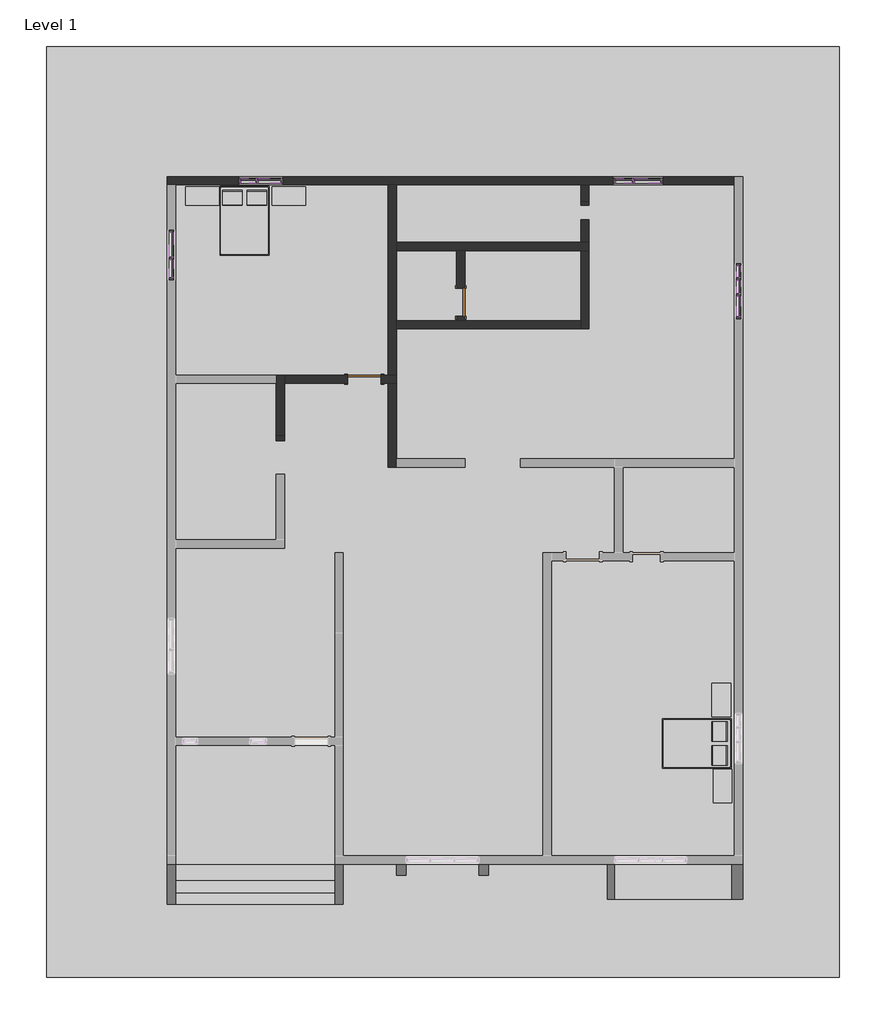
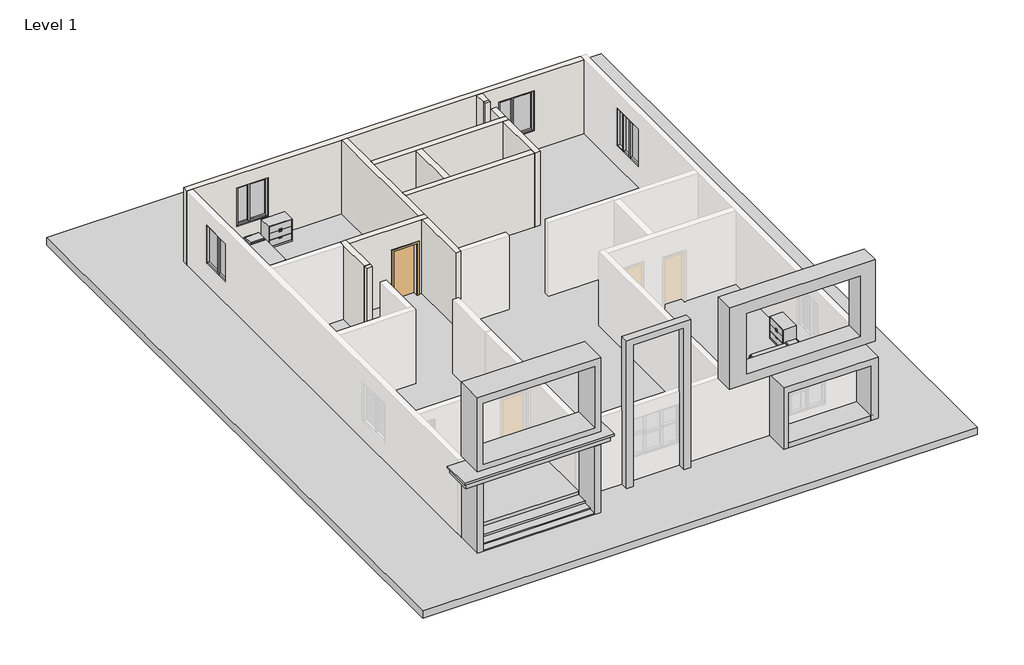
# One storey, part 3 of 3: 31 members, 13 walls, 9 plates, 6 furniture elements, 3 proxies, 2 doors.
"""IFC4 building model written with IfcOpenShell, lengths in millimetres."""

from ifc_helpers import new_model, si_unit, frame, origin, origin_with_axes, place, context, project, spatial, polyline, outline, extrude, faceted_brep, transform, mapped, element, save
from components import generic_models_1_generic_models_1_3e26791c, generic_models_2_generic_models_2_3b55f561, generic_models_3_generic_models_3_0a189295, door_a1484949, door_0ca8825f, furniture_b58f7881, furniture_dccb195e, member_6f432376, member_b9f3750b, member_83c59054, member_02b8d6b6, member_8456be0a, member_cf38170e, member_5535eeb3, member_7007ad49, member_f01f4494, member_224a2a57, member_3f0e0172, member_dc106669, member_0b703233, member_623289aa, member_5f1d7e17, member_11644e99, member_f1c24713, system_panel_glazed_ed2eb233, system_panel_glazed_a8d9a87a, system_panel_glazed_d172bbbe, system_panel_glazed_c29ca9bc, system_panel_glazed_863e5c36, system_panel_glazed_5eb5e9ea, system_panel_glazed_fad1f0ba, system_panel_glazed_bca51d21, system_panel_glazed_cf012afc

model = new_model("IFC4")

# Units and contexts
model_context = context("Model", 3, world=origin())
ifc_project = project(units=[si_unit("LENGTHUNIT", "METRE", prefix="MILLI")], contexts=[model_context])

# Site, building, storey
site = spatial("IfcSite", under=ifc_project)
building = spatial("IfcBuilding", under=site)
storey = spatial("IfcBuildingStorey", under=building, Name="Level 1", Elevation=0.0)

# Proxies
placement = place(None, origin())
generic_models_1_generic_models_1_shape = generic_models_1_generic_models_1_3e26791c(model_context)
element("IfcBuildingElementProxy", 1, Name="Generic Models 1 : Generic Models 1", ObjectType="Generic Models 1 : Generic Models 1", at=placement, inside=storey, context=model_context, shape_type="MappedRepresentation", body=[
    mapped(generic_models_1_generic_models_1_shape, transform((0.0, 0.0, 0.0), x_axis=(1.0, 0.0, 0.0), y_axis=(0.0, 1.0, 0.0), z_axis=(0.0, 0.0, 1.0))),
])
generic_models_2_generic_models_2_shape = generic_models_2_generic_models_2_3b55f561(model_context)
element("IfcBuildingElementProxy", 2, Name="Generic Models 2 : Generic Models 2", ObjectType="Generic Models 2 : Generic Models 2", at=placement, inside=storey, context=model_context, shape_type="MappedRepresentation", body=[
    mapped(generic_models_2_generic_models_2_shape, transform((0.0, 0.0, 0.0), x_axis=(1.0, 0.0, 0.0), y_axis=(0.0, 1.0, 0.0), z_axis=(0.0, 0.0, 1.0))),
])
generic_models_3_generic_models_3_shape = generic_models_3_generic_models_3_0a189295(model_context)
element("IfcBuildingElementProxy", 3, Name="Generic Models 3 : Generic Models 3", ObjectType="Generic Models 3 : Generic Models 3", at=placement, inside=storey, context=model_context, shape_type="MappedRepresentation", body=[
    mapped(generic_models_3_generic_models_3_shape, transform((0.0, 0.0, 0.0), x_axis=(1.0, 0.0, 0.0), y_axis=(0.0, 1.0, 0.0), z_axis=(0.0, 0.0, 1.0))),
])

# Doors
door_shape = door_a1484949(model_context)
element("IfcDoor", 4, ObjectType="Single-Flush : 30\" x 80\"", at=placement, inside=storey, context=model_context, shape_type="MappedRepresentation", body=[
    mapped(door_shape, transform((-11084.7702714, 3728.4616097, 0.0), x_axis=(0.0, -1.0, 0.0), y_axis=(1.0, 0.0, 0.0), z_axis=(0.0, 0.0, 1.0))),
])
door_2_shape = door_0ca8825f(model_context)
element("IfcDoor", 5, ObjectType="Single-Flush : 36\" x 84\"", at=placement, inside=storey, context=model_context, shape_type="MappedRepresentation", body=[
    mapped(door_2_shape, transform((-13713.6702714, 1632.9616097, 0.0), x_axis=(1.0, 0.0, 0.0), y_axis=(0.0, 1.0, 0.0), z_axis=(0.0, 0.0, 1.0))),
])

# Furniture
furniture_shape = furniture_b58f7881(model_context)
element("IfcFurniture", 6, ObjectType="Bed-Box : Double 53\" x 74\"", at=placement, inside=storey, context=model_context, shape_type="MappedRepresentation", body=[
    mapped(furniture_shape, transform((-17316.7227304, 6185.3911179, 0.0), x_axis=(1.0, 0.0, 0.0), y_axis=(0.0, 1.0, 0.0), z_axis=(0.0, 0.0, 1.0))),
])
element("IfcFurniture", 7, ObjectType="Bed-Box : Double 53\" x 74\"", at=placement, inside=storey, context=model_context, shape_type="MappedRepresentation", body=[
    mapped(furniture_shape, transform((-4411.4407632, -7959.2859313, 0.0), x_axis=(0.0, -1.0, 0.0), y_axis=(1.0, 0.0, 0.0), z_axis=(0.0, 0.0, 1.0))),
])
furniture_2_shape = furniture_dccb195e(model_context)
element("IfcFurniture", 8, ObjectType="Cabinet File-Lateral 3 Drawer : 36\" x 20\" x 36\"", at=placement, inside=storey, context=model_context, shape_type="MappedRepresentation", body=[
    mapped(furniture_2_shape, transform((-3038.4518953, -7284.6609042, 0.0), x_axis=(0.0, -1.0, 0.0), y_axis=(1.0, 0.0, 0.0), z_axis=(0.0, 0.0, 1.0))),
])
element("IfcFurniture", 9, ObjectType="Cabinet File-Lateral 3 Drawer : 36\" x 20\" x 36\"", at=placement, inside=storey, context=model_context, shape_type="MappedRepresentation", body=[
    mapped(furniture_2_shape, transform((-3000.3518953, -9634.1609042, 0.0), x_axis=(0.0, -1.0, 0.0), y_axis=(1.0, 0.0, 0.0), z_axis=(0.0, 0.0, 1.0))),
])
element("IfcFurniture", 10, ObjectType="Cabinet File-Lateral 3 Drawer : 36\" x 20\" x 36\"", at=placement, inside=storey, context=model_context, shape_type="MappedRepresentation", body=[
    mapped(furniture_2_shape, transform((-15591.0477575, 7558.3799858, 0.0), x_axis=(1.0, 0.0, 0.0), y_axis=(0.0, 1.0, 0.0), z_axis=(0.0, 0.0, 1.0))),
])
element("IfcFurniture", 11, ObjectType="Cabinet File-Lateral 3 Drawer : 36\" x 20\" x 36\"", at=placement, inside=storey, context=model_context, shape_type="MappedRepresentation", body=[
    mapped(furniture_2_shape, transform((-17953.2477575, 7558.3799858, 0.0), x_axis=(1.0, 0.0, 0.0), y_axis=(0.0, 1.0, 0.0), z_axis=(0.0, 0.0, 1.0))),
])

# Members
member_shape = member_6f432376(model_context)
element("IfcMember", 12, ObjectType="Rectangular Mullion : 2.5\" x 5\" rectangular", at=placement, inside=storey, context=model_context, shape_type="MappedRepresentation", body=[
    mapped(member_shape, transform((-3502.8702714, 3334.7616097, 2404.522235), x_axis=(0.0, 0.0, 1.0), y_axis=(-1.0, 0.0, 0.0), z_axis=(0.0, -1.0, 0.0))),
])
element("IfcMember", 13, ObjectType="Rectangular Mullion : 2.5\" x 5\" rectangular", at=placement, inside=storey, context=model_context, shape_type="MappedRepresentation", body=[
    mapped(member_shape, transform((-3502.8702714, 3899.9116097, 784.7381643), x_axis=(0.0, 0.0, -1.0), y_axis=(-1.0, 0.0, 0.0), z_axis=(0.0, 1.0, 0.0))),
])
member_2_shape = member_b9f3750b(model_context)
element("IfcMember", 14, ObjectType="Rectangular Mullion : 2.5\" x 5\" rectangular", at=placement, inside=storey, context=model_context, shape_type="MappedRepresentation", body=[
    mapped(member_2_shape, transform((-18971.4702714, 4890.5116097, 810.1702203), x_axis=(0.0, 0.0, -1.0), y_axis=(-1.0, 0.0, 0.0), z_axis=(0.0, 1.0, 0.0))),
])
element("IfcMember", 15, ObjectType="Rectangular Mullion : 2.5\" x 5\" rectangular", at=placement, inside=storey, context=model_context, shape_type="MappedRepresentation", body=[
    mapped(member_2_shape, transform((-18971.4702714, 4401.5616097, 2441.6213003), x_axis=(0.0, 0.0, 1.0), y_axis=(-1.0, 0.0, 0.0), z_axis=(0.0, -1.0, 0.0))),
])
member_3_shape = member_83c59054(model_context)
element("IfcMember", 16, ObjectType="Rectangular Mullion : 2.5\" x 5\" rectangular", at=placement, inside=storey, context=model_context, shape_type="MappedRepresentation", body=[
    mapped(member_3_shape, transform((-3502.8702714, 4331.7116097, 784.7381643), x_axis=(0.0, 0.0, -1.0), y_axis=(-1.0, 0.0, 0.0), z_axis=(0.0, 1.0, 0.0))),
])
member_4_shape = member_02b8d6b6(model_context)
element("IfcMember", 17, ObjectType="Rectangular Mullion : 2.5\" x 5\" rectangular", at=placement, inside=storey, context=model_context, shape_type="MappedRepresentation", body=[
    mapped(member_4_shape, transform((-3502.8702714, 4731.7616097, 784.7381643), x_axis=(0.0, 0.0, -1.0), y_axis=(-1.0, 0.0, 0.0), z_axis=(0.0, 1.0, 0.0))),
])
member_5_shape = member_8456be0a(model_context)
element("IfcMember", 18, ObjectType="Rectangular Mullion : 2.5\" x 5\" rectangular", at=placement, inside=storey, context=model_context, shape_type="MappedRepresentation", body=[
    mapped(member_5_shape, transform((-3502.8702714, 3931.6616097, 784.7381643), x_axis=(0.0, -1.0, 0.0), y_axis=(-1.0, 0.0, 0.0), z_axis=(0.0, 0.0, -1.0))),
])
element("IfcMember", 19, ObjectType="Rectangular Mullion : 2.5\" x 5\" rectangular", at=placement, inside=storey, context=model_context, shape_type="MappedRepresentation", body=[
    mapped(member_5_shape, transform((-3502.8702714, 4363.4616097, 784.7381643), x_axis=(0.0, -1.0, 0.0), y_axis=(-1.0, 0.0, 0.0), z_axis=(0.0, 0.0, -1.0))),
])
element("IfcMember", 20, ObjectType="Rectangular Mullion : 2.5\" x 5\" rectangular", at=placement, inside=storey, context=model_context, shape_type="MappedRepresentation", body=[
    mapped(member_4_shape, transform((-3502.8702714, 4395.2116097, 2404.522235), x_axis=(0.0, 0.0, 1.0), y_axis=(-1.0, 0.0, 0.0), z_axis=(0.0, -1.0, 0.0))),
])
element("IfcMember", 21, ObjectType="Rectangular Mullion : 2.5\" x 5\" rectangular", at=placement, inside=storey, context=model_context, shape_type="MappedRepresentation", body=[
    mapped(member_3_shape, transform((-3502.8702714, 3963.4116097, 2404.522235), x_axis=(0.0, 0.0, 1.0), y_axis=(-1.0, 0.0, 0.0), z_axis=(0.0, -1.0, 0.0))),
])
member_6_shape = member_cf38170e(model_context)
element("IfcMember", 22, ObjectType="Rectangular Mullion : 2.5\" x 5\" rectangular", at=placement, inside=storey, context=model_context, shape_type="MappedRepresentation", body=[
    mapped(member_6_shape, transform((-3502.8702714, 4795.2616097, 2404.522235), x_axis=(0.0, 1.0, 0.0), y_axis=(-1.0, 0.0, 0.0), z_axis=(0.0, 0.0, 1.0))),
])
element("IfcMember", 23, ObjectType="Rectangular Mullion : 2.5\" x 5\" rectangular", at=placement, inside=storey, context=model_context, shape_type="MappedRepresentation", body=[
    mapped(member_6_shape, transform((-3502.8702714, 3271.2616097, 784.7381643), x_axis=(0.0, -1.0, 0.0), y_axis=(-1.0, 0.0, 0.0), z_axis=(0.0, 0.0, -1.0))),
])
member_7_shape = member_5535eeb3(model_context)
element("IfcMember", 24, ObjectType="Rectangular Mullion : 2.5\" x 5\" rectangular", at=placement, inside=storey, context=model_context, shape_type="MappedRepresentation", body=[
    mapped(member_7_shape, transform((-6404.8202714, 7043.1616097, 2451.8488146), x_axis=(0.0, 0.0, 1.0), y_axis=(0.0, -1.0, 0.0), z_axis=(1.0, 0.0, 0.0))),
])
member_8_shape = member_7007ad49(model_context)
element("IfcMember", 25, ObjectType="Rectangular Mullion : 2.5\" x 5\" rectangular", at=placement, inside=storey, context=model_context, shape_type="MappedRepresentation", body=[
    mapped(member_8_shape, transform((-5623.7702714, 7043.1616097, 2451.8488146), x_axis=(0.0, 0.0, 1.0), y_axis=(0.0, -1.0, 0.0), z_axis=(1.0, 0.0, 0.0))),
])
member_9_shape = member_f01f4494(model_context)
element("IfcMember", 26, ObjectType="Rectangular Mullion : 2.5\" x 5\" rectangular", at=placement, inside=storey, context=model_context, shape_type="MappedRepresentation", body=[
    mapped(member_9_shape, transform((-6373.0702714, 7043.1616097, 795.4375908), x_axis=(1.0, 0.0, 0.0), y_axis=(0.0, -1.0, 0.0), z_axis=(0.0, 0.0, -1.0))),
])
element("IfcMember", 27, ObjectType="Rectangular Mullion : 2.5\" x 5\" rectangular", at=placement, inside=storey, context=model_context, shape_type="MappedRepresentation", body=[
    mapped(member_8_shape, transform((-6341.3202714, 7043.1616097, 795.4375908), x_axis=(0.0, 0.0, -1.0), y_axis=(0.0, -1.0, 0.0), z_axis=(-1.0, 0.0, 0.0))),
])
element("IfcMember", 28, ObjectType="Rectangular Mullion : 2.5\" x 5\" rectangular", at=placement, inside=storey, context=model_context, shape_type="MappedRepresentation", body=[
    mapped(member_7_shape, transform((-6868.3702714, 7043.1616097, 795.4375908), x_axis=(0.0, 0.0, -1.0), y_axis=(0.0, -1.0, 0.0), z_axis=(-1.0, 0.0, 0.0))),
])
member_10_shape = member_224a2a57(model_context)
element("IfcMember", 29, ObjectType="Rectangular Mullion : 2.5\" x 5\" rectangular", at=placement, inside=storey, context=model_context, shape_type="MappedRepresentation", body=[
    mapped(member_10_shape, transform((-6931.8702714, 7043.1616097, 2451.8488146), x_axis=(-1.0, 0.0, 0.0), y_axis=(0.0, -1.0, 0.0), z_axis=(0.0, 0.0, 1.0))),
])
element("IfcMember", 30, ObjectType="Rectangular Mullion : 2.5\" x 5\" rectangular", at=placement, inside=storey, context=model_context, shape_type="MappedRepresentation", body=[
    mapped(member_10_shape, transform((-5560.2702714, 7043.1616097, 795.4375908), x_axis=(1.0, 0.0, 0.0), y_axis=(0.0, -1.0, 0.0), z_axis=(0.0, 0.0, -1.0))),
])
member_11_shape = member_3f0e0172(model_context)
element("IfcMember", 31, ObjectType="Rectangular Mullion : 2.5\" x 5\" rectangular", at=placement, inside=storey, context=model_context, shape_type="MappedRepresentation", body=[
    mapped(member_11_shape, transform((-16602.9202714, 7043.1616097, 907.4058093), x_axis=(0.0, 0.0, -1.0), y_axis=(0.0, -1.0, 0.0), z_axis=(-1.0, 0.0, 0.0))),
])
member_12_shape = member_dc106669(model_context)
element("IfcMember", 32, ObjectType="Rectangular Mullion : 2.5\" x 5\" rectangular", at=placement, inside=storey, context=model_context, shape_type="MappedRepresentation", body=[
    mapped(member_12_shape, transform((-17079.1702714, 7043.1616097, 907.4058093), x_axis=(0.0, 0.0, -1.0), y_axis=(0.0, -1.0, 0.0), z_axis=(-1.0, 0.0, 0.0))),
])
member_13_shape = member_0b703233(model_context)
element("IfcMember", 33, ObjectType="Rectangular Mullion : 2.5\" x 5\" rectangular", at=placement, inside=storey, context=model_context, shape_type="MappedRepresentation", body=[
    mapped(member_13_shape, transform((-16634.6702714, 7043.1616097, 907.4058093), x_axis=(1.0, 0.0, 0.0), y_axis=(0.0, -1.0, 0.0), z_axis=(0.0, 0.0, -1.0))),
])
element("IfcMember", 34, ObjectType="Rectangular Mullion : 2.5\" x 5\" rectangular", at=placement, inside=storey, context=model_context, shape_type="MappedRepresentation", body=[
    mapped(member_12_shape, transform((-16666.4202714, 7043.1616097, 2493.6914356), x_axis=(0.0, 0.0, 1.0), y_axis=(0.0, -1.0, 0.0), z_axis=(1.0, 0.0, 0.0))),
])
element("IfcMember", 35, ObjectType="Rectangular Mullion : 2.5\" x 5\" rectangular", at=placement, inside=storey, context=model_context, shape_type="MappedRepresentation", body=[
    mapped(member_11_shape, transform((-15986.9702714, 7043.1616097, 2493.6914356), x_axis=(0.0, 0.0, 1.0), y_axis=(0.0, -1.0, 0.0), z_axis=(1.0, 0.0, 0.0))),
])
member_14_shape = member_623289aa(model_context)
element("IfcMember", 36, ObjectType="Rectangular Mullion : 2.5\" x 5\" rectangular", at=placement, inside=storey, context=model_context, shape_type="MappedRepresentation", body=[
    mapped(member_14_shape, transform((-17142.6702714, 7043.1616097, 2493.6914356), x_axis=(-1.0, 0.0, 0.0), y_axis=(0.0, -1.0, 0.0), z_axis=(0.0, 0.0, 1.0))),
])
element("IfcMember", 37, ObjectType="Rectangular Mullion : 2.5\" x 5\" rectangular", at=placement, inside=storey, context=model_context, shape_type="MappedRepresentation", body=[
    mapped(member_14_shape, transform((-15923.4702714, 7043.1616097, 907.4058093), x_axis=(1.0, 0.0, 0.0), y_axis=(0.0, -1.0, 0.0), z_axis=(0.0, 0.0, -1.0))),
])
member_15_shape = member_5f1d7e17(model_context)
element("IfcMember", 38, ObjectType="Rectangular Mullion : 2.5\" x 5\" rectangular", at=placement, inside=storey, context=model_context, shape_type="MappedRepresentation", body=[
    mapped(member_15_shape, transform((-18971.4702714, 4954.0116097, 2441.6213003), x_axis=(0.0, 0.0, 1.0), y_axis=(-1.0, 0.0, 0.0), z_axis=(0.0, -1.0, 0.0))),
])
member_16_shape = member_11644e99(model_context)
element("IfcMember", 39, ObjectType="Rectangular Mullion : 2.5\" x 5\" rectangular", at=placement, inside=storey, context=model_context, shape_type="MappedRepresentation", body=[
    mapped(member_16_shape, transform((-18971.4702714, 4922.2616097, 810.1702203), x_axis=(0.0, -1.0, 0.0), y_axis=(-1.0, 0.0, 0.0), z_axis=(0.0, 0.0, -1.0))),
])
element("IfcMember", 40, ObjectType="Rectangular Mullion : 2.5\" x 5\" rectangular", at=placement, inside=storey, context=model_context, shape_type="MappedRepresentation", body=[
    mapped(member_15_shape, transform((-18971.4702714, 5646.1616097, 810.1702203), x_axis=(0.0, 0.0, -1.0), y_axis=(-1.0, 0.0, 0.0), z_axis=(0.0, 1.0, 0.0))),
])
member_17_shape = member_f1c24713(model_context)
element("IfcMember", 41, ObjectType="Rectangular Mullion : 2.5\" x 5\" rectangular", at=placement, inside=storey, context=model_context, shape_type="MappedRepresentation", body=[
    mapped(member_17_shape, transform((-18971.4702714, 4338.0616097, 810.1702203), x_axis=(0.0, -1.0, 0.0), y_axis=(-1.0, 0.0, 0.0), z_axis=(0.0, 0.0, -1.0))),
])
element("IfcMember", 42, ObjectType="Rectangular Mullion : 2.5\" x 5\" rectangular", at=placement, inside=storey, context=model_context, shape_type="MappedRepresentation", body=[
    mapped(member_17_shape, transform((-18971.4702714, 5709.6616097, 2441.6213003), x_axis=(0.0, 1.0, 0.0), y_axis=(-1.0, 0.0, 0.0), z_axis=(0.0, 0.0, 1.0))),
])

# Plates
system_panel_glazed_shape = system_panel_glazed_ed2eb233(model_context)
element("IfcPlate", 43, ObjectType="System Panel : Glazed", at=placement, inside=storey, context=model_context, shape_type="MappedRepresentation", body=[
    mapped(system_panel_glazed_shape, transform((-3502.8702714, 4563.4866097, 848.2381643), x_axis=(0.0, -1.0, 0.0), y_axis=(1.0, 0.0, 0.0), z_axis=(0.0, 0.0, 1.0))),
])
system_panel_glazed_2_shape = system_panel_glazed_a8d9a87a(model_context)
element("IfcPlate", 44, ObjectType="System Panel : Glazed", at=placement, inside=storey, context=model_context, shape_type="MappedRepresentation", body=[
    mapped(system_panel_glazed_2_shape, transform((-3502.8702714, 3617.3366097, 848.2381643), x_axis=(0.0, -1.0, 0.0), y_axis=(1.0, 0.0, 0.0), z_axis=(0.0, 0.0, 1.0))),
])
system_panel_glazed_3_shape = system_panel_glazed_d172bbbe(model_context)
element("IfcPlate", 45, ObjectType="System Panel : Glazed", at=placement, inside=storey, context=model_context, shape_type="MappedRepresentation", body=[
    mapped(system_panel_glazed_3_shape, transform((-3502.8702714, 4147.5616097, 848.2381643), x_axis=(0.0, -1.0, 0.0), y_axis=(1.0, 0.0, 0.0), z_axis=(0.0, 0.0, 1.0))),
])
system_panel_glazed_4_shape = system_panel_glazed_c29ca9bc(model_context)
element("IfcPlate", 46, ObjectType="System Panel : Glazed", at=placement, inside=storey, context=model_context, shape_type="MappedRepresentation", body=[
    mapped(system_panel_glazed_4_shape, transform((-6636.5952714, 7043.1616097, 858.9375908), x_axis=(1.0, 0.0, 0.0), y_axis=(0.0, 1.0, 0.0), z_axis=(0.0, 0.0, 1.0))),
])
system_panel_glazed_5_shape = system_panel_glazed_863e5c36(model_context)
element("IfcPlate", 47, ObjectType="System Panel : Glazed", at=placement, inside=storey, context=model_context, shape_type="MappedRepresentation", body=[
    mapped(system_panel_glazed_5_shape, transform((-5982.5452714, 7043.1616097, 858.9375908), x_axis=(1.0, 0.0, 0.0), y_axis=(0.0, 1.0, 0.0), z_axis=(0.0, 0.0, 1.0))),
])
system_panel_glazed_6_shape = system_panel_glazed_5eb5e9ea(model_context)
element("IfcPlate", 48, ObjectType="System Panel : Glazed", at=placement, inside=storey, context=model_context, shape_type="MappedRepresentation", body=[
    mapped(system_panel_glazed_6_shape, transform((-16872.7952714, 7043.1616097, 970.9058093), x_axis=(1.0, 0.0, 0.0), y_axis=(0.0, 1.0, 0.0), z_axis=(0.0, 0.0, 1.0))),
])
system_panel_glazed_7_shape = system_panel_glazed_fad1f0ba(model_context)
element("IfcPlate", 49, ObjectType="System Panel : Glazed", at=placement, inside=storey, context=model_context, shape_type="MappedRepresentation", body=[
    mapped(system_panel_glazed_7_shape, transform((-16294.9452714, 7043.1616097, 970.9058093), x_axis=(1.0, 0.0, 0.0), y_axis=(0.0, 1.0, 0.0), z_axis=(0.0, 0.0, 1.0))),
])
system_panel_glazed_8_shape = system_panel_glazed_bca51d21(model_context)
element("IfcPlate", 50, ObjectType="System Panel : Glazed", at=placement, inside=storey, context=model_context, shape_type="MappedRepresentation", body=[
    mapped(system_panel_glazed_8_shape, transform((-18971.4702714, 5300.0866097, 873.6702203), x_axis=(0.0, -1.0, 0.0), y_axis=(1.0, 0.0, 0.0), z_axis=(0.0, 0.0, 1.0))),
])
system_panel_glazed_9_shape = system_panel_glazed_cf012afc(model_context)
element("IfcPlate", 51, ObjectType="System Panel : Glazed", at=placement, inside=storey, context=model_context, shape_type="MappedRepresentation", body=[
    mapped(system_panel_glazed_9_shape, transform((-18971.4702714, 4646.0366097, 873.6702203), x_axis=(0.0, -1.0, 0.0), y_axis=(1.0, 0.0, 0.0), z_axis=(0.0, 0.0, 1.0))),
])

# Walls
element("IfcWall", 52, ObjectType="9\"", at=placement, inside=storey, context=model_context, shape_type="Brep", body=[
    faceted_brep([(-3617.1702714, 7157.4616097, 0.0), (-19085.7702714, 7157.4616097, 0.0), (-19085.7702714, 7157.4616097, 3048.0), (-3617.1702714, 7157.4616097, 3048.0), (-6931.8702714, 7157.4616097, 2451.8488146), (-6931.8702714, 7157.4616097, 795.4375908), (-5560.2702714, 7157.4616097, 795.4375908), (-5560.2702714, 7157.4616097, 2451.8488146), (-17142.6702714, 7157.4616097, 2493.6914356), (-17142.6702714, 7157.4616097, 907.4058093), (-15923.4702714, 7157.4616097, 907.4058093), (-15923.4702714, 7157.4616097, 2493.6914356), (-19085.7702714, 6928.8616097, 0.0), (-18857.1702714, 6928.8616097, 0.0), (-13065.9702714, 6928.8616097, 0.0), (-12837.3702714, 6928.8616097, 0.0), (-7808.1702714, 6928.8616097, 0.0), (-7579.5702714, 6928.8616097, 0.0), (-3617.1702714, 6928.8616097, 0.0), (-3617.1702714, 6928.8616097, 3048.0), (-7579.5702714, 6928.8616097, 3048.0), (-7808.1702714, 6928.8616097, 3048.0), (-12837.3702714, 6928.8616097, 3048.0), (-13065.9702714, 6928.8616097, 3048.0), (-18857.1702714, 6928.8616097, 3048.0), (-19085.7702714, 6928.8616097, 3048.0), (-6931.8702714, 6928.8616097, 795.4375908), (-6931.8702714, 6928.8616097, 2451.8488146), (-5560.2702714, 6928.8616097, 2451.8488146), (-5560.2702714, 6928.8616097, 795.4375908), (-17142.6702714, 6928.8616097, 907.4058093), (-17142.6702714, 6928.8616097, 2493.6914356), (-15923.4702714, 6928.8616097, 2493.6914356), (-15923.4702714, 6928.8616097, 907.4058093)], [[[0, 1, 2, 3], [4, 5, 6, 7], [8, 9, 10, 11]], [[12, 13, 14, 15, 16, 17, 18, 19, 20, 21, 22, 23, 24, 25], [26, 27, 28, 29], [30, 31, 32, 33]], [[1, 0, 18, 17, 16, 15, 14, 13, 12]], [[3, 2, 25, 24, 23, 22, 21, 20, 19]], [[0, 3, 19, 18]], [[2, 1, 12, 25]], [[4, 27, 26, 5]], [[27, 4, 7, 28]], [[28, 7, 6, 29]], [[5, 26, 29, 6]], [[30, 9, 8, 31]], [[31, 8, 11, 32]], [[32, 11, 10, 33]], [[9, 30, 33, 10]]]),
])
element("IfcWall", 53, ObjectType="9\"", at=placement, inside=storey, context=model_context, shape_type="Brep", body=[
    faceted_brep([(-13256.4702714, 1518.6616097, 2133.6), (-13256.4702714, 1518.6616097, 0.0), (-13065.9702714, 1518.6616097, 0.0), (-12837.3702714, 1518.6616097, 0.0), (-12837.3702714, 1518.6616097, 3048.0), (-13065.9702714, 1518.6616097, 3048.0), (-15885.3702714, 1518.6616097, 3048.0), (-15885.3702714, 1518.6616097, 0.0), (-14170.8702714, 1518.6616097, 0.0), (-14170.8702714, 1518.6616097, 2133.6), (-12837.3702714, 1747.2616097, 0.0), (-13065.9702714, 1747.2616097, 0.0), (-13256.4702714, 1747.2616097, 0.0), (-13256.4702714, 1747.2616097, 2133.6), (-14170.8702714, 1747.2616097, 2133.6), (-14170.8702714, 1747.2616097, 0.0), (-15885.3702714, 1747.2616097, 0.0), (-15885.3702714, 1747.2616097, 3048.0), (-13065.9702714, 1747.2616097, 3048.0), (-12837.3702714, 1747.2616097, 3048.0)], [[[0, 1, 2, 3, 4, 5, 6, 7, 8, 9]], [[10, 11, 12, 13, 14, 15, 16, 17, 18, 19]], [[8, 7, 16, 15]], [[3, 2, 1, 12, 11, 10]], [[6, 5, 4, 19, 18, 17]], [[7, 6, 17, 16]], [[4, 3, 10, 19]], [[13, 12, 1, 0]], [[14, 13, 0, 9]], [[15, 14, 9, 8]]]),
])
element("IfcWall", 54, ObjectType="9\"", at=placement, inside=storey, context=model_context, shape_type="Brep", body=[
    faceted_brep([(-12837.3702714, 1747.2616097, 0.0), (-12837.3702714, 3004.5616097, 0.0), (-12837.3702714, 3233.1616097, 0.0), (-12837.3702714, 5138.1616097, 0.0), (-12837.3702714, 5366.7616097, 0.0), (-12837.3702714, 6928.8616097, 0.0), (-12837.3702714, 6928.8616097, 3048.0), (-12837.3702714, 5366.7616097, 3048.0), (-12837.3702714, 5138.1616097, 3048.0), (-12837.3702714, 3233.1616097, 3048.0), (-12837.3702714, 3004.5616097, 3048.0), (-12837.3702714, 1747.2616097, 3048.0), (-13065.9702714, 1747.2616097, 0.0), (-13065.9702714, 1747.2616097, 3048.0), (-13065.9702714, 6928.8616097, 3048.0), (-13065.9702714, 6928.8616097, 0.0)], [[[0, 1, 2, 3, 4, 5, 6, 7, 8, 9, 10, 11]], [[12, 13, 14, 15]], [[5, 4, 3, 2, 1, 0, 12, 15]], [[11, 10, 9, 8, 7, 6, 14, 13]], [[0, 11, 13, 12]], [[6, 5, 15, 14]]]),
])
element("IfcWall", 55, ObjectType="9\"", at=placement, inside=storey, context=model_context, shape_type="Brep", body=[
    faceted_brep([(-12837.3702714, 5138.1616097, 0.0), (-11199.0702714, 5138.1616097, 0.0), (-10970.4702714, 5138.1616097, 0.0), (-7808.1702714, 5138.1616097, 0.0), (-7579.5702714, 5138.1616097, 0.0), (-7579.5702714, 5138.1616097, 3048.0), (-7808.1702714, 5138.1616097, 3048.0), (-10970.4702714, 5138.1616097, 3048.0), (-11199.0702714, 5138.1616097, 3048.0), (-12837.3702714, 5138.1616097, 3048.0), (-12837.3702714, 5366.7616097, 0.0), (-12837.3702714, 5366.7616097, 3048.0), (-7808.1702714, 5366.7616097, 3048.0), (-7579.5702714, 5366.7616097, 3048.0), (-7579.5702714, 5366.7616097, 0.0), (-7808.1702714, 5366.7616097, 0.0)], [[[0, 1, 2, 3, 4, 5, 6, 7, 8, 9]], [[10, 11, 12, 13, 14, 15]], [[4, 3, 2, 1, 0, 10, 15, 14]], [[9, 8, 7, 6, 5, 13, 12, 11]], [[0, 9, 11, 10]], [[5, 4, 14, 13]]]),
])
element("IfcWall", 56, ObjectType="9\"", at=placement, inside=storey, context=model_context, shape_type="SweptSolid", body=[
    extrude(outline(polyline([(-7579.5702714, 5976.3616097), (-7579.5702714, 5366.7616097), (-7808.1702714, 5366.7616097), (-7808.1702714, 5976.3616097), (-7579.5702714, 5976.3616097)])), origin_with_axes(), (0.0, 0.0, 1.0), 3048.0),
])
element("IfcWall", 57, ObjectType="9\"", at=placement, inside=storey, context=model_context, shape_type="Brep", body=[
    faceted_brep([(-13065.9702714, 1518.6616097, 0.0), (-13065.9702714, -767.3383903, 0.0), (-13065.9702714, -767.3383903, 3048.0), (-13065.9702714, 1518.6616097, 3048.0), (-12837.3702714, 1518.6616097, 0.0), (-12837.3702714, 1518.6616097, 3048.0), (-12837.3702714, -538.7383903, 3048.0), (-12837.3702714, -767.3383903, 3048.0), (-12837.3702714, -767.3383903, 0.0), (-12837.3702714, -538.7383903, 0.0)], [[[0, 1, 2, 3]], [[4, 5, 6, 7, 8, 9]], [[1, 0, 4, 9, 8]], [[3, 2, 7, 6, 5]], [[0, 3, 5, 4]], [[2, 1, 8, 7]]]),
])
element("IfcWall", 58, ObjectType="9\"", at=placement, inside=storey, context=model_context, shape_type="Brep", body=[
    faceted_brep([(-7808.1702714, 5138.1616097, 0.0), (-7808.1702714, 3233.1616097, 0.0), (-7808.1702714, 3004.5616097, 0.0), (-7808.1702714, 3004.5616097, 3048.0), (-7808.1702714, 3233.1616097, 3048.0), (-7808.1702714, 5138.1616097, 3048.0), (-7579.5702714, 5138.1616097, 0.0), (-7579.5702714, 5138.1616097, 3048.0), (-7579.5702714, 3004.5616097, 3048.0), (-7579.5702714, 3004.5616097, 0.0)], [[[0, 1, 2, 3, 4, 5]], [[6, 7, 8, 9]], [[2, 1, 0, 6, 9]], [[5, 4, 3, 8, 7]], [[0, 5, 7, 6]], [[3, 2, 9, 8]]]),
])
element("IfcWall", 59, ObjectType="9\"", at=placement, inside=storey, context=model_context, shape_type="Brep", body=[
    faceted_brep([(-7808.1702714, 3233.1616097, 0.0), (-10970.4702714, 3233.1616097, 0.0), (-11199.0702714, 3233.1616097, 0.0), (-12837.3702714, 3233.1616097, 0.0), (-12837.3702714, 3233.1616097, 3048.0), (-11199.0702714, 3233.1616097, 3048.0), (-10970.4702714, 3233.1616097, 3048.0), (-7808.1702714, 3233.1616097, 3048.0), (-7808.1702714, 3004.5616097, 0.0), (-7808.1702714, 3004.5616097, 3048.0), (-12837.3702714, 3004.5616097, 3048.0), (-12837.3702714, 3004.5616097, 0.0)], [[[0, 1, 2, 3, 4, 5, 6, 7]], [[8, 9, 10, 11]], [[3, 2, 1, 0, 8, 11]], [[7, 6, 5, 4, 10, 9]], [[0, 7, 9, 8]], [[4, 3, 11, 10]]]),
])
element("IfcWall", 60, ObjectType="9\"", at=placement, inside=storey, context=model_context, shape_type="SweptSolid", body=[
    extrude(outline(polyline([(3347.4616097, 2032.0), (3347.4616097, 0.0), (3233.1616097, 0.0), (3233.1616097, 3048.0), (5138.1616097, 3048.0), (5138.1616097, 0.0), (4109.4616097, 0.0), (4109.4616097, 2032.0), (3347.4616097, 2032.0)])), frame((-11199.0702714, 0.0, 0.0), z_axis=(1.0, 0.0, 0.0), x_axis=(0.0, 1.0, 0.0)), (0.0, 0.0, 1.0), 228.6),
])
element("IfcWall", 61, ObjectType="9\"", at=placement, inside=storey, context=model_context, shape_type="Brep", body=[
    faceted_brep([(-15885.3702714, 108.9616097, 0.0), (-15885.3702714, 1518.6616097, 0.0), (-15885.3702714, 1747.2616097, 0.0), (-15885.3702714, 1747.2616097, 3048.0), (-15885.3702714, 1518.6616097, 3048.0), (-15885.3702714, 108.9616097, 3048.0), (-16113.9702714, 108.9616097, 0.0), (-16113.9702714, 108.9616097, 3048.0), (-16113.9702714, 1518.6616097, 3048.0), (-16113.9702714, 1747.2616097, 3048.0), (-16113.9702714, 1747.2616097, 0.0), (-16113.9702714, 1518.6616097, 0.0)], [[[0, 1, 2, 3, 4, 5]], [[6, 7, 8, 9, 10, 11]], [[2, 1, 0, 6, 11, 10]], [[5, 4, 3, 9, 8, 7]], [[0, 5, 7, 6]], [[3, 2, 10, 9]]]),
])
element("IfcWall", 62, ObjectType="9\"", at=placement, inside=storey, context=model_context, shape_type="SweptSolid", body=[
    extrude(outline(polyline([(-15885.3702714, 108.9616097), (-15885.3702714, -43.4383903), (-16113.9702714, -43.4383903), (-16113.9702714, 108.9616097), (-15885.3702714, 108.9616097)])), origin_with_axes(), (0.0, 0.0, 1.0), 3048.0),
])
element("IfcWall", 63, ObjectType="9\"", at=placement, inside=storey, context=model_context, shape_type="SweptSolid", body=[
    extrude(outline(polyline([(-7579.5702714, 6928.8616097), (-7579.5702714, 6484.3616097), (-7808.1702714, 6484.3616097), (-7808.1702714, 6928.8616097), (-7579.5702714, 6928.8616097)])), origin_with_axes(), (0.0, 0.0, 1.0), 3048.0),
])
element("IfcWall", 64, ObjectType="9\"", at=placement, inside=storey, context=model_context, shape_type="SweptSolid", body=[
    extrude(outline(polyline([(-7579.5702714, 6484.3616097), (-7579.5702714, 6382.7616097), (-7808.1702714, 6382.7616097), (-7808.1702714, 6484.3616097), (-7579.5702714, 6484.3616097)])), origin_with_axes(), (0.0, 0.0, 1.0), 3048.0),
])

save(model, "model.ifc")

# Revit data of these elements
# Type "Single-Flush : 30\" x 80\""
#   Type Mark = "5"
#   Construction Type Id = "MDOOR"
#   Assembly Code = "C1020"
#   Analytic Construction = "Metal"
#   Thickness = 0' - 2"
#   Heat Transfer Coefficient (U) = 0.651978 BTU/(h·ft²·°F)
#   Height = 6' - 8"
#   Trim Projection Ext = 0' - 1"
#   Trim Projection Int = 0' - 1"
#   Trim Width = 0' - 3"
#   Width = 2' - 6"
#   Define Thermal Properties by = 1
#   Define Thermal Properties by = 1
#   Door Material = Door - Panel
#   Frame Material = Door - Frame
#   Visual Light Transmittance = 0
#   Solar Heat Gain Coefficient = 0
#   Function = (empty or 0)
#   Wall Closure = (empty or 0)
# Type "Single-Flush : 36\" x 84\""
#   Type Mark = "1"
#   Construction Type Id = "MDOOR"
#   Assembly Code = "C1020"
#   Analytic Construction = "Metal"
#   Thickness = 0' - 2"
#   Heat Transfer Coefficient (U) = 0.651978 BTU/(h·ft²·°F)
#   Height = 7' - 0"
#   Trim Projection Ext = 0' - 1"
#   Trim Projection Int = 0' - 1"
#   Trim Width = 0' - 3"
#   Width = 3' - 0"
#   Define Thermal Properties by = 1
#   Define Thermal Properties by = 1
#   Door Material = Door - Panel
#   Frame Material = Door - Frame
#   Visual Light Transmittance = 0
#   Solar Heat Gain Coefficient = 0
#   Function = (empty or 0)
#   Wall Closure = (empty or 0)
# Type "Bed-Box : Double 53\" x 74\""
#   Assembly Code = "E2020200"
#   Length = 6' - 2"
#   Width = 4' - 5"
#   Frame Material = Birch
#   Mattress Material = Linen, White
#   Default Elevation = 0
# Type "Cabinet File-Lateral 3 Drawer : 36\" x 20\" x 36\""
#   Assembly Code = "E2020200"
#   Depth = 1' - 8"
#   Height = 3' - 0"
#   Width = 3' - 0"
#   Material = Metal - Steel
#   Default Elevation = 0
# Type "Rectangular Mullion : 2.5\" x 5\" rectangular"
#   built-in parameter 1007304 = 0.416667 (stored number, unit not read)
#   built-in parameter 1007301 = 0.104167 (stored number, unit not read)
#   built-in parameter 1007300 = 0.104167 (stored number, unit not read)
# Type "System Panel : Glazed"
#   Construction Type Id = "GSP4R"
#   Analytic Construction = "1/8 in Pilkington single glazing"
#   Visual Light Transmittance = 0.9
#   Solar Heat Gain Coefficient = 0.86
#   Heat Transfer Coefficient (U) = 1.18115 BTU/(h·ft²·°F)
#   Define Thermal Properties by = 1
# Type "9\""
#   Assembly Code = "B2010"
#   Layers, outside or top first: 0' - 9" no material (function 1)
# Element 1 (IfcBuildingElementProxy, "Generic Models 1 : Generic Models 1")
#   Phase Created = New Construction
# Element 2 (IfcBuildingElementProxy, "Generic Models 2 : Generic Models 2")
#   Phase Created = New Construction
# Element 3 (IfcBuildingElementProxy, "Generic Models 3 : Generic Models 3")
#   Phase Created = New Construction
# Element 4 (IfcDoor, "Single-Flush : 30\" x 80\"")
#   Phase Created = New Construction
#   Materials on its faces: "Door - Frame", "Door - Panel"
# Element 5 (IfcDoor, "Single-Flush : 36\" x 84\"")
#   Phase Created = New Construction
#   Materials on its faces: "Door - Frame", "Door - Panel"
# Elements 6, 7 (IfcFurniture, "Bed-Box : Double 53\" x 74\"")
#   Phase Created = New Construction
#   Materials on its faces: "Birch", "Linen, White"
# Elements 8, 9, 10, 11 (IfcFurniture, "Cabinet File-Lateral 3 Drawer : 36\" x 20\" x 36\"")
#   Phase Created = New Construction
#   Materials on its faces: "Metal - Steel"
# Elements 12, 13, 14, 15, 16, 17, 18, 19, 20, 21, 22, 23, 24, 25, 26, 27, 28, 29, 30, 31, 32, 33, 34, 35, 36, 37, 38, 39, 40, 41, 42 (IfcMember, "Rectangular Mullion : 2.5\" x 5\" rectangular")
#   Phase Created = New Construction
#   Materials on its faces: "Aluminum"
# Elements 43, 44, 45, 46, 47, 48, 49, 50, 51 (IfcPlate, "System Panel : Glazed")
#   Phase Created = New Construction
#   Materials on its faces: "Glass"
# Elements 52, 53, 54, 55, 56, 57, 58, 59, 60, 61, 62, 63, 64 (IfcWall, "9\"")
#   Top Offset = 0' - 0"
#   Base Offset = 0' - 0"
#   Unconnected Height = 10' - 0"
#   wall height = 10' - 0"
#   Phase Created = New Construction
#   Base Constraint = Level 1
#   Materials on its faces: "Default Wall"
# Materials
#   "Door - Panel": class "Wood", colour RGB 210 159 95, transparency 0, Cost = 0
#   "Door - Frame": colour RGB 118 70 51, transparency 0, Cost = 0
#   "Birch": class "Wood", colour RGB 224 178 126, transparency 0, Description = "Betula Alleghaniensis", Cost = 0
#   "Linen, White": class "Textile", colour RGB 247 247 239, transparency 0, Description = "Linen, white", Cost = 0
#   "Metal - Steel": colour RGB 209 209 209, transparency 0
#   "Aluminum": class "Metal", colour RGB 247 247 247, transparency 0, Description = "Aluminum 6061", Cost = 0
#   "Glass": class "Glass", colour RGB 0 128 192, transparency 0.75, Description = "Soda Lime Glass", Cost = 0
#   "Default Wall": colour RGB 128 128 128, transparency 0, Cost = 0
